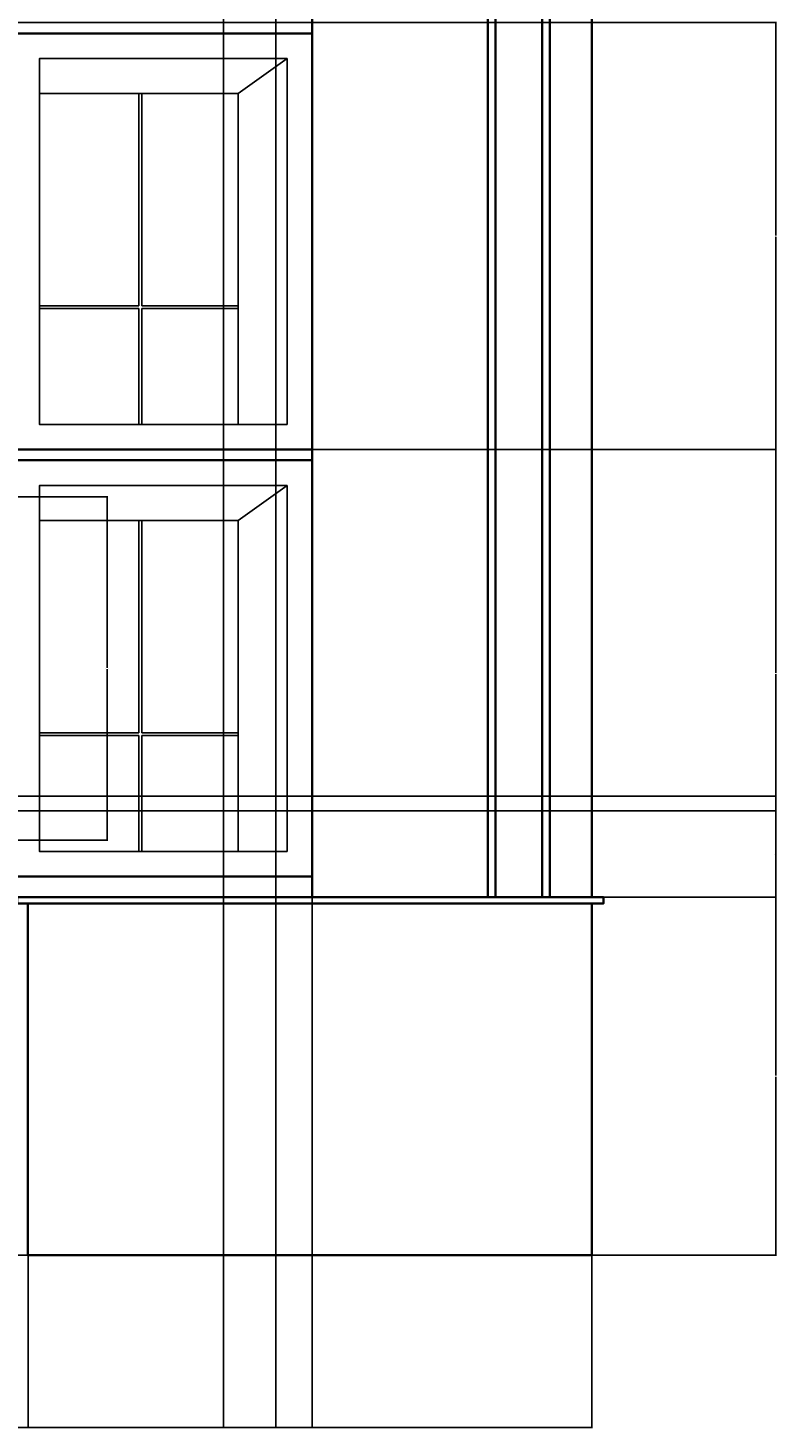
# Model space of a CAD drawing. Units: feet. Extents: x 1141 to 2858, y 751 to 1654.
# Tile 10 of 13: x 2621 to 2858, y 751 to 1195. Entities that reach past the tile are written whole.
import ezdxf

# ---------------------------------------------------------------- set-up
doc = ezdxf.new("R2010")
doc.units = ezdxf.units.FT
for name, color, linetype, lineweight in [('A-ANNO-DIMS', 2, 'Continuous', 18), ('A-ELEV', 7, 'Continuous', 35), ('A-ELEV-PATT', 8, 'Continuous', 13), ('A-GLAZ', 4, 'Continuous', 25)]:
    doc.layers.add(name, color=color, linetype=linetype, lineweight=lineweight)
doc.styles.get("Standard").update_dxf_attribs({"font": 'arial.ttf'})
doc.dimstyles.get("Standard").update_dxf_attribs({"dimtxt": 0.18, "dimasz": 0.18, "dimexe": 0.18, "dimexo": 0.0625, "dimgap": 0.09, "dimtad": 0, "dimtih": 1, "dimtoh": 1, "dimdec": 1, "dimzin": 0, "dimdsep": 46, "dimlunit": 3, "dimtxsty": 'Standard', "dimcen": 0.09, "dimadec": 0, "dimazin": 0, "dimtfac": 1, "dimtdec": 1, "dimtofl": 0, "dimtmove": 0, "dimatfit": 3, "dimfxl": 1, "dimtolj": 1, "dimtzin": 0, "dimarcsym": 0})

# ---------------------------------------------------------------- blocks, each defined once
blk = doc.blocks.new('WIN-SIDE-B')
blk.add_line((63.09, 104.94), (78.57, 116.03))
blk.add_lwpolyline([(78.57, 0), (0, 0), (0, 116.03), (78.57, 116.03)], close=True)
for points in [[(63.09, 0), (63.09, 104.94), (0, 104.94)], [(31.54, 37.61), (31.54, 104.94), (32.46, 104.94), (32.46, 37.61)], [(31.54, 36.79), (0, 36.79), (0, 37.61), (31.54, 37.61)], [(32.46, 36.79), (32.46, 0), (31.54, 0), (31.54, 36.79)], [(32.46, 37.61), (63.09, 37.61), (63.09, 36.79), (32.46, 36.79)]]:
    blk.add_lwpolyline(points)
blk = doc.blocks.new('*D21')
at = {"layer": 'A-ANNO-DIMS', "color": 0, "lineweight": -2, "transparency": 16777216}
for p, q in [((2604.62, 1046.32), (2645.79, 1046.32)), ((2645.61, 1046.14), (2645.61, 992.08)), ((2645.61, 937.66), (2645.61, 991.72)), ((2604.62, 937.48), (2645.79, 937.48))]:
    blk.add_line(p, q, dxfattribs=at)
at = {"layer": 'A-ANNO-DIMS', "color": 0, "transparency": 16777216}
for points in [[(2645.58, 1046.14), (2645.64, 1046.14), (2645.61, 1046.32)], [(2645.58, 937.66), (2645.64, 937.66), (2645.61, 937.48)]]:
    blk.add_solid(points, dxfattribs=at)
at = {"layer": 'Defpoints', "color": 0, "transparency": 16777216}
for p in [(2604.56, 1046.32), (2645.61, 1046.32), (2604.56, 937.48)]:
    blk.add_point(p, dxfattribs=at)
at = {"layer": 'A-ANNO-DIMS', "color": 0, "transparency": 16777216, "insert": (2645.61, 991.9), "char_height": 0.18, "attachment_point": 5}
blk.add_mtext('\\A1;109 TYP.', dxfattribs=at)
blk = doc.blocks.new('*D29')
at = {"layer": 'A-ANNO-DIMS', "color": 0, "lineweight": -2, "transparency": 16777216}
for p, q in [((2206.09, 919.34), (2857.83, 919.34)), ((2857.65, 919.16), (2857.65, 862.8)), ((2857.65, 806.08), (2857.65, 862.44)), ((2206.09, 805.9), (2857.83, 805.9))]:
    blk.add_line(p, q, dxfattribs=at)
at = {"layer": 'A-ANNO-DIMS', "color": 0, "transparency": 16777216}
for points in [[(2857.62, 919.16), (2857.68, 919.16), (2857.65, 919.34)], [(2857.62, 806.08), (2857.68, 806.08), (2857.65, 805.9)]]:
    blk.add_solid(points, dxfattribs=at)
at = {"layer": 'Defpoints', "color": 0, "transparency": 16777216}
for p in [(2206.03, 919.34), (2857.65, 919.34), (2206.03, 805.9)]:
    blk.add_point(p, dxfattribs=at)
at = {"layer": 'A-ANNO-DIMS', "color": 0, "transparency": 16777216, "insert": (2857.65, 862.62), "char_height": 0.18, "attachment_point": 5}
blk.add_mtext('\\A1;113.44', dxfattribs=at)
blk = doc.blocks.new('*D30')
at = {"layer": 'A-ANNO-DIMS', "color": 0, "lineweight": -2, "transparency": 16777216}
for p, q in [((2117.47, 1061.29), (2857.83, 1061.29)), ((2857.65, 1061.11), (2857.65, 990.5)), ((2857.65, 919.52), (2857.65, 990.13)), ((2117.47, 919.34), (2857.83, 919.34))]:
    blk.add_line(p, q, dxfattribs=at)
at = {"layer": 'A-ANNO-DIMS', "color": 0, "transparency": 16777216}
for points in [[(2857.62, 1061.11), (2857.68, 1061.11), (2857.65, 1061.29)], [(2857.62, 919.52), (2857.68, 919.52), (2857.65, 919.34)]]:
    blk.add_solid(points, dxfattribs=at)
at = {"layer": 'Defpoints', "color": 0, "transparency": 16777216}
for p in [(2117.41, 1061.29), (2857.65, 1061.29), (2117.41, 919.34)]:
    blk.add_point(p, dxfattribs=at)
at = {"layer": 'A-ANNO-DIMS', "color": 0, "transparency": 16777216, "insert": (2857.65, 990.31), "char_height": 0.18, "attachment_point": 5}
blk.add_mtext('\\A1;141.95', dxfattribs=at)
blk = doc.blocks.new('*D31')
at = {"layer": 'A-ANNO-DIMS', "color": 0, "lineweight": -2, "transparency": 16777216}
for p, q in [((2117.47, 1196.68), (2857.83, 1196.68)), ((2857.65, 1196.5), (2857.65, 1129.16)), ((2857.65, 1061.47), (2857.65, 1128.8)), ((2117.47, 1061.29), (2857.83, 1061.29))]:
    blk.add_line(p, q, dxfattribs=at)
at = {"layer": 'A-ANNO-DIMS', "color": 0, "transparency": 16777216}
for points in [[(2857.62, 1196.5), (2857.68, 1196.5), (2857.65, 1196.68)], [(2857.62, 1061.47), (2857.68, 1061.47), (2857.65, 1061.29)]]:
    blk.add_solid(points, dxfattribs=at)
at = {"layer": 'Defpoints', "color": 0, "transparency": 16777216}
for p in [(2117.41, 1196.68), (2857.65, 1196.68), (2117.41, 1061.29)]:
    blk.add_point(p, dxfattribs=at)
at = {"layer": 'A-ANNO-DIMS', "color": 0, "transparency": 16777216, "insert": (2857.65, 1128.98), "char_height": 0.18, "attachment_point": 5}
blk.add_mtext('\\A1;135.4', dxfattribs=at)
blk = doc.blocks.new('*D37')
at = {"layer": 'A-ANNO-DIMS', "color": 0, "lineweight": -2, "transparency": 16777216}
for p, q in [((2445.45, 805.84), (2445.45, 751.07)), ((2620.53, 805.84), (2620.53, 751.07)), ((2445.63, 751.25), (2532.53, 751.25)), ((2620.35, 751.25), (2533.44, 751.25))]:
    blk.add_line(p, q, dxfattribs=at)
at = {"layer": 'A-ANNO-DIMS', "color": 0, "transparency": 16777216}
for points in [[(2445.63, 751.28), (2445.63, 751.22), (2445.45, 751.25)], [(2620.35, 751.28), (2620.35, 751.22), (2620.53, 751.25)]]:
    blk.add_solid(points, dxfattribs=at)
at = {"layer": 'Defpoints', "color": 0, "transparency": 16777216}
for p in [(2445.45, 805.9), (2620.53, 805.9), (2620.53, 751.25)]:
    blk.add_point(p, dxfattribs=at)
at = {"layer": 'A-ANNO-DIMS', "color": 0, "transparency": 16777216, "insert": (2532.99, 751.25), "char_height": 0.18, "attachment_point": 5}
blk.add_mtext('\\A1;175.08', dxfattribs=at)
blk = doc.blocks.new('*D38')
at = {"layer": 'A-ANNO-DIMS', "color": 0, "lineweight": -2, "transparency": 16777216}
for p, q in [((2620.53, 805.84), (2620.53, 751.07)), ((2799.3, 805.84), (2799.3, 751.07)), ((2620.71, 751.25), (2709.46, 751.25)), ((2799.12, 751.25), (2710.37, 751.25))]:
    blk.add_line(p, q, dxfattribs=at)
at = {"layer": 'A-ANNO-DIMS', "color": 0, "transparency": 16777216}
for points in [[(2620.71, 751.28), (2620.71, 751.22), (2620.53, 751.25)], [(2799.12, 751.28), (2799.12, 751.22), (2799.3, 751.25)]]:
    blk.add_solid(points, dxfattribs=at)
at = {"layer": 'Defpoints', "color": 0, "transparency": 16777216}
for p in [(2620.53, 805.9), (2799.3, 805.9), (2799.3, 751.25)]:
    blk.add_point(p, dxfattribs=at)
at = {"layer": 'A-ANNO-DIMS', "color": 0, "transparency": 16777216, "insert": (2709.91, 751.25), "char_height": 0.18, "attachment_point": 5}
blk.add_mtext('\\A1;178.77', dxfattribs=at)
blk = doc.blocks.new('*D41')
at = {"layer": 'A-ANNO-DIMS', "color": 0, "lineweight": -2, "transparency": 16777216}
for p, q in [((2616.14, 1193.23), (2616.14, 751.07)), ((2710.68, 1193.23), (2710.68, 751.07)), ((2616.32, 751.25), (2663.01, 751.25)), ((2710.5, 751.25), (2663.8, 751.25))]:
    blk.add_line(p, q, dxfattribs=at)
at = {"layer": 'A-ANNO-DIMS', "color": 0, "transparency": 16777216}
for points in [[(2616.32, 751.28), (2616.32, 751.22), (2616.14, 751.25)], [(2710.5, 751.28), (2710.5, 751.22), (2710.68, 751.25)]]:
    blk.add_solid(points, dxfattribs=at)
at = {"layer": 'Defpoints', "color": 0, "transparency": 16777216}
for p in [(2616.14, 1193.29), (2710.68, 1193.29), (2710.68, 751.25)]:
    blk.add_point(p, dxfattribs=at)
at = {"layer": 'A-ANNO-DIMS', "color": 0, "transparency": 16777216, "insert": (2663.41, 751.25), "char_height": 0.18, "attachment_point": 5}
blk.add_mtext('\\A1;94.54', dxfattribs=at)
blk = doc.blocks.new('*D71')
at = {"layer": 'A-ANNO-DIMS', "color": 0, "lineweight": -2, "transparency": 16777216}
for p, q in [((2682.47, 1352.88), (2682.47, 751.07)), ((2699.1, 1343.58), (2699.1, 751.07)), ((2682.65, 751.25), (2690.4, 751.25)), ((2698.92, 751.25), (2691.17, 751.25))]:
    blk.add_line(p, q, dxfattribs=at)
at = {"layer": 'A-ANNO-DIMS', "color": 0, "transparency": 16777216}
for points in [[(2682.65, 751.28), (2682.65, 751.22), (2682.47, 751.25)], [(2698.92, 751.28), (2698.92, 751.22), (2699.1, 751.25)]]:
    blk.add_solid(points, dxfattribs=at)
at = {"layer": 'Defpoints', "color": 0, "transparency": 16777216}
for p in [(2682.47, 1352.94), (2699.1, 1343.65), (2699.1, 751.25)]:
    blk.add_point(p, dxfattribs=at)
at = {"layer": 'A-ANNO-DIMS', "color": 0, "transparency": 16777216, "insert": (2690.78, 751.25), "char_height": 0.18, "attachment_point": 5}
blk.add_mtext('\\A1;16.63', dxfattribs=at)
blk = doc.blocks.new('*D72')
at = {"layer": 'A-ANNO-DIMS', "color": 0, "lineweight": -2, "transparency": 16777216}
for p, q in [((2699.1, 1343.58), (2699.1, 751.07)), ((2710.68, 1332), (2710.68, 751.07)), ((2699.28, 751.25), (2704.5, 751.25)), ((2710.5, 751.25), (2705.27, 751.25))]:
    blk.add_line(p, q, dxfattribs=at)
at = {"layer": 'A-ANNO-DIMS', "color": 0, "transparency": 16777216}
for points in [[(2699.28, 751.28), (2699.28, 751.22), (2699.1, 751.25)], [(2710.5, 751.28), (2710.5, 751.22), (2710.68, 751.25)]]:
    blk.add_solid(points, dxfattribs=at)
at = {"layer": 'Defpoints', "color": 0, "transparency": 16777216}
for p in [(2699.1, 1343.65), (2710.68, 1332.06), (2710.68, 751.25)]:
    blk.add_point(p, dxfattribs=at)
at = {"layer": 'A-ANNO-DIMS', "color": 0, "transparency": 16777216, "insert": (2704.89, 751.25), "char_height": 0.18, "attachment_point": 5}
blk.add_mtext('\\A1;11.58', dxfattribs=at)
blk = doc.blocks.new('*D74')
at = {"layer": 'A-ANNO-DIMS', "color": 0, "lineweight": -2, "transparency": 16777216}
for p, q in [((2413.84, 1332), (2413.84, 751.07)), ((2710.68, 1332), (2710.68, 751.07)), ((2414.02, 751.25), (2561.79, 751.25)), ((2710.5, 751.25), (2562.72, 751.25))]:
    blk.add_line(p, q, dxfattribs=at)
at = {"layer": 'A-ANNO-DIMS', "color": 0, "transparency": 16777216}
for points in [[(2414.02, 751.28), (2414.02, 751.22), (2413.84, 751.25)], [(2710.5, 751.28), (2710.5, 751.22), (2710.68, 751.25)]]:
    blk.add_solid(points, dxfattribs=at)
at = {"layer": 'Defpoints', "color": 0, "transparency": 16777216}
for p in [(2413.84, 1332.06), (2710.68, 1332.06), (2710.68, 751.25)]:
    blk.add_point(p, dxfattribs=at)
at = {"layer": 'A-ANNO-DIMS', "color": 0, "transparency": 16777216, "insert": (2562.26, 751.25), "char_height": 0.18, "attachment_point": 5}
blk.add_mtext('\\A1;296.83', dxfattribs=at)
blk = doc.blocks.new('*D80')
at = {"layer": 'A-ANNO-DIMS', "color": 0, "lineweight": -2, "transparency": 16777216}
for p, q in [((2347.57, 946.77), (2857.83, 946.77)), ((2857.65, 946.59), (2857.65, 933.24)), ((2857.65, 919.52), (2857.65, 932.87)), ((2319.36, 919.34), (2857.83, 919.34))]:
    blk.add_line(p, q, dxfattribs=at)
at = {"layer": 'A-ANNO-DIMS', "color": 0, "transparency": 16777216}
for points in [[(2857.62, 946.59), (2857.68, 946.59), (2857.65, 946.77)], [(2857.62, 919.52), (2857.68, 919.52), (2857.65, 919.34)]]:
    blk.add_solid(points, dxfattribs=at)
at = {"layer": 'Defpoints', "color": 0, "transparency": 16777216}
for p in [(2347.51, 946.77), (2857.65, 946.77), (2319.3, 919.34)]:
    blk.add_point(p, dxfattribs=at)
at = {"layer": 'A-ANNO-DIMS', "color": 0, "transparency": 16777216, "insert": (2857.65, 933.06), "char_height": 0.18, "attachment_point": 5}
blk.add_mtext('\\A1;27.435', dxfattribs=at)
blk = doc.blocks.new('*D81')
at = {"layer": 'A-ANNO-DIMS', "color": 0, "lineweight": -2, "transparency": 16777216}
for p, q in [((2525.7, 951.43), (2857.83, 951.43)), ((2857.65, 951.25), (2857.65, 935.57)), ((2857.65, 919.52), (2857.65, 935.2)), ((2319.36, 919.34), (2857.83, 919.34))]:
    blk.add_line(p, q, dxfattribs=at)
at = {"layer": 'A-ANNO-DIMS', "color": 0, "transparency": 16777216}
for points in [[(2857.62, 951.25), (2857.68, 951.25), (2857.65, 951.43)], [(2857.62, 919.52), (2857.68, 919.52), (2857.65, 919.34)]]:
    blk.add_solid(points, dxfattribs=at)
at = {"layer": 'Defpoints', "color": 0, "transparency": 16777216}
for p in [(2525.64, 951.43), (2857.65, 951.43), (2319.3, 919.34)]:
    blk.add_point(p, dxfattribs=at)
at = {"layer": 'A-ANNO-DIMS', "color": 0, "transparency": 16777216, "insert": (2857.65, 935.38), "char_height": 0.18, "attachment_point": 5}
blk.add_mtext('\\A1;32.09', dxfattribs=at)

msp = doc.modelspace()

# ---------------------------------------------------------------- hatches: boundary and pattern name
at = {"layer": 'A-ELEV-PATT'}
h = msp.add_hatch(color=256, dxfattribs=at)
h.dxf.hatch_style = 1
h.paths.add_polyline_path([(1812.5866, 1456.0789), (1734.0179, 1456.0789), (1749.501, 1444.9949), (1812.5866, 1444.9949)], flags=0)
h.paths.add_polyline_path([(1820.5724, 1464.0647), (1726.032, 1464.0647), (1726.032, 1332.0647), (1820.5724, 1332.0647)])
h.paths.add_polyline_path([(1734.0179, 1456.0789), (1812.5866, 1456.0789), (1812.5866, 1340.0506), (1734.0179, 1340.0506)], flags=16)
h.paths.add_polyline_path([(1749.501, 1444.9949), (1781.0438, 1444.9949), (1781.0438, 1377.6615), (1812.5866, 1377.6615), (1812.5866, 1376.842), (1781.0438, 1376.842), (1781.0438, 1340.0506), (1780.1289, 1340.0506), (1780.1289, 1376.842), (1749.501, 1376.842), (1749.501, 1377.6615)], flags=0)
h.paths.add_polyline_path([(1749.501, 1444.9949), (1734.0179, 1456.0789), (1734.0179, 1340.0506), (1749.501, 1340.0506)], flags=0)
h.paths.add_polyline_path([(1820.5724, 1328.6768), (1726.032, 1328.6768), (1726.032, 1196.6768), (1820.5724, 1196.6768)])
h.paths.add_polyline_path([(1734.0179, 1320.6909), (1812.5866, 1320.6909), (1812.5866, 1204.6626), (1734.0179, 1204.6626)], flags=16)
h.paths.add_polyline_path([(1749.501, 1309.6069), (1781.0438, 1309.6069), (1781.0438, 1242.2735), (1812.5866, 1242.2735), (1812.5866, 1241.454), (1781.0438, 1241.454), (1781.0438, 1204.6626), (1780.1289, 1204.6626), (1780.1289, 1241.454), (1749.501, 1241.454), (1749.501, 1242.2735)], flags=0)
h.paths.add_polyline_path([(1749.501, 1309.6069), (1734.0179, 1320.6909), (1734.0179, 1204.6626), (1749.501, 1204.6626)], flags=0)
h.paths.add_polyline_path([(2117.407, 1193.2888), (2022.8666, 1193.2888), (2022.8666, 1061.2888), (2117.407, 1061.2888)])
h.paths.add_polyline_path([(2109.4211, 1185.3029), (2109.4211, 1069.2747), (2030.8524, 1069.2747), (2030.8524, 1185.3029)], flags=16)
h.paths.add_polyline_path([(2093.938, 1174.219), (2093.938, 1106.066), (2063.3101, 1106.066), (2063.3101, 1069.2747), (2062.3952, 1069.2747), (2062.3952, 1106.066), (2030.8524, 1106.066), (2030.8524, 1106.8855), (2062.3952, 1106.8855), (2062.3952, 1174.219), (2063.3101, 1174.219)], flags=0)
h.paths.add_polyline_path([(2702.6903, 1049.9149), (2624.1217, 1049.9149), (2624.1217, 1038.831), (2687.2072, 1038.831), (2687.2072, 933.8867), (2702.6903, 933.8867)], flags=0)
h.paths.add_polyline_path([(2109.4211, 1049.9149), (2093.938, 1038.831), (2093.938, 933.8867), (2109.4211, 933.8867)])
h.paths.add_polyline_path([(2109.4211, 1049.9149), (2030.8524, 1049.9149), (2030.8524, 1038.831), (2093.938, 1038.831)])

# ---------------------------------------------------------------- linework, layer by layer
at = {"layer": 'A-ELEV'}
for p, q in [((2710.6762, 1057.9008), (2319.3013, 1057.9008)), ((2319.3013, 925.9008), (2710.6762, 925.9008))]:
    msp.add_line(p, q, dxfattribs=at)
for points in [[(2799.3013, 919.339), (2799.3013, 1599.4527), (2710.6762, 1599.4527), (2710.6762, 919.339)], [(2768.7322, 919.339), (2768.7322, 1599.4527), (2766.2848, 1599.4527), (2766.2848, 919.339)], [(2785.9583, 919.339), (2785.9583, 1599.4527), (2783.5108, 1599.4527), (2783.5108, 919.339)], [(2710.6762, 917.3598), (2799.3013, 917.3598)], [(2766.2848, 917.3598), (2768.7322, 917.3598)], [(2783.5108, 917.3598), (2785.9583, 917.3598)]]:
    msp.add_lwpolyline(points, dxfattribs=at)
for points in [[(2710.6762, 1061.2888), (2616.1358, 1061.2888), (2616.1358, 1193.2888), (2710.6762, 1193.2888)], [(2710.6762, 925.9008), (2616.1358, 925.9008), (2616.1358, 1057.9008), (2710.6762, 1057.9008)], [(2617.048, 917.3598), (2802.9989, 917.3598), (2802.9989, 919.339), (2617.048, 919.339)], [(2799.3013, 805.9008), (2620.5281, 805.9008), (2620.5281, 917.3598), (2799.3013, 917.3598)]]:
    msp.add_lwpolyline(points, close=True, dxfattribs=at)

# ---------------------------------------------------------------- block references
at = {"layer": 'A-GLAZ'}
for p in [(2624.122, 1069.2751), (2624.122, 933.8871)]:
    msp.add_blockref('WIN-SIDE-B', p, dxfattribs=at)

# ---------------------------------------------------------------- dimensions: what is measured, and where the dimension line sits
at = {"layer": 'A-ANNO-DIMS'}
for base, p1, p2, picture, middle in [((2699.0959, 751.2508), (2682.4659, 1352.9376), (2699.0959, 1343.645), '*D71', (2690.7809, 751.2508)), ((2710.6762, 751.2508), (2699.0959, 1343.645), (2710.6762, 1332.0647), '*D72', (2704.886, 751.2508)), ((2710.6762, 751.2508), (2413.8417, 1332.0647), (2710.6762, 1332.0647), '*D74', (2562.2589, 751.2508)), ((2710.6762, 751.2508), (2616.1358, 1193.2888), (2710.6762, 1193.2888), '*D41', (2663.406, 751.2508)), ((2620.5281, 751.2508), (2445.4463, 805.9008), (2620.5281, 805.9008), '*D37', (2532.9872, 751.2508)), ((2799.3013, 751.2508), (2620.5281, 805.9008), (2799.3013, 805.9008), '*D38', (2709.9147, 751.2508))]:
    dim = msp.add_linear_dim(base=base, p1=p1, p2=p2, dimstyle='Standard', override={"dimdec": 2, "dimlfac": 1, "dimrnd": 0, "dimzin": 0, "dimdsep": 46, "dimlunit": 2}, dxfattribs=at)
    dim.commit()
    dim.dimension.update_dxf_attribs({"geometry": picture, "text_midpoint": middle})
for base, p1, p2, override, picture, middle in [((2857.6489, 1196.6768), (2117.407, 1061.2888), (2117.407, 1196.6768), {"dimdec": 1, "dimlfac": 1, "dimrnd": 0, "dimzin": 0, "dimdsep": 46, "dimlunit": 2}, '*D31', (2857.6489, 1128.9828)), ((2857.6489, 1061.2888), (2117.407, 919.339), (2117.407, 1061.2888), {"dimdec": 2, "dimlfac": 1, "dimrnd": 0, "dimzin": 0, "dimdsep": 46, "dimlunit": 2}, '*D30', (2857.6489, 990.3139)), ((2857.6489, 951.4297), (2319.3013, 919.339), (2525.6422, 951.4297), {"dimdec": 2, "dimlfac": 1, "dimrnd": 0, "dimzin": 0, "dimdsep": 46, "dimlunit": 2}, '*D81', (2857.6489, 935.3843)), ((2857.6489, 946.7736), (2319.3013, 919.339), (2347.5116, 946.7736), {"dimdec": 3, "dimlfac": 1, "dimrnd": 0, "dimzin": 0, "dimdsep": 46, "dimlunit": 2}, '*D80', (2857.6489, 933.0563)), ((2857.6489, 919.339), (2206.032, 805.9008), (2206.032, 919.339), {"dimdec": 2, "dimlfac": 1, "dimrnd": 0, "dimzin": 0, "dimdsep": 46, "dimlunit": 2}, '*D29', (2857.6489, 862.6199))]:
    dim = msp.add_linear_dim(base=base, p1=p1, p2=p2, angle=90, dimstyle='Standard', override=override, dxfattribs=at)
    dim.commit()
    dim.dimension.update_dxf_attribs({"geometry": picture, "text_midpoint": middle})
dim = msp.add_linear_dim(base=(2645.6066, 1046.3205), p1=(2604.5555, 937.4811), p2=(2604.5555, 1046.3205), angle=90, text='<> TYP.', dimstyle='Standard', override={"dimdec": 0, "dimlfac": 1, "dimrnd": 0, "dimzin": 0, "dimdsep": 46, "dimlunit": 2}, dxfattribs=at)
dim.commit()
dim.dimension.update_dxf_attribs({"geometry": '*D21', "text_midpoint": (2645.6066, 991.9008)})

doc.saveas('drawing.dxf')
